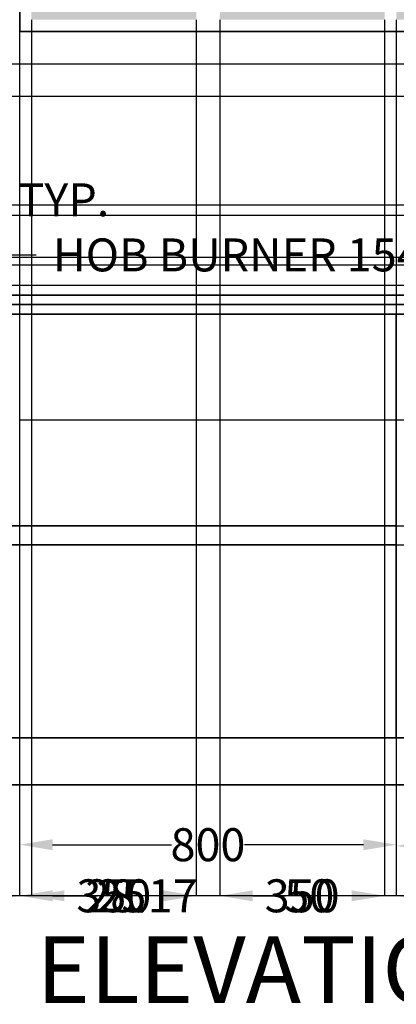
# Model space of a CAD drawing. Units: inches. Extents: x 600 to 5582, y -464 to 3142.
# Tile 7 of 9: x 3385 to 4185, y -464 to 1627. Entities that reach past the tile are written whole.
import ezdxf

# ---------------------------------------------------------------- set-up
doc = ezdxf.new("R2010")
doc.units = ezdxf.units.IN
doc.header["$MEASUREMENT"] = 0
for name, color, linetype, lineweight in [('A-ANNO-DIMS', 2, 'Continuous', 18), ('A-ANNO-TEXT', 7, 'Continuous', 25), ('A-ELEV', 7, 'Continuous', 35), ('A-ELEV-PATT', 252, 'Continuous', 13)]:
    doc.layers.add(name, color=color, linetype=linetype, lineweight=lineweight)
doc.styles.get("Standard").update_dxf_attribs({"font": 'arial.ttf'})
doc.dimstyles.get("Standard").update_dxf_attribs({"dimtxt": 70, "dimasz": 70, "dimexe": 0.18, "dimexo": 0.0625, "dimgap": 0.09, "dimtad": 0, "dimtih": 1, "dimtoh": 1, "dimdec": 0, "dimzin": 0, "dimdsep": 46, "dimtxsty": 'Standard', "dimcen": 0.09, "dimadec": 0, "dimazin": 0, "dimtfac": 1, "dimtdec": 0, "dimtofl": 0, "dimtmove": 0, "dimatfit": 3, "dimfxl": 1, "dimtolj": 1, "dimtzin": 0, "dimarcsym": 0})

# ---------------------------------------------------------------- blocks, each defined once
blk = doc.blocks.new('*D13')
at = {"layer": 'A-ANNO-DIMS', "color": 0, "lineweight": -2, "transparency": 16777216}
for p, q in [((3384.7, 2.4), (3384.7, -124.8)), ((4184.7, 2.4), (4184.7, -124.8)), ((3454.7, -124.6), (3707.4, -124.6)), ((4114.7, -124.6), (3862.1, -124.6))]:
    blk.add_line(p, q, dxfattribs=at)
at = {"layer": 'A-ANNO-DIMS', "color": 0, "transparency": 16777216}
for points in [[(3454.7, -113), (3454.7, -136.3), (3384.7, -124.6)], [(4114.7, -113), (4114.7, -136.3), (4184.7, -124.6)]]:
    blk.add_solid(points, dxfattribs=at)
at = {"layer": 'Defpoints', "color": 0, "transparency": 16777216}
for p in [(3384.7, 2.4), (4184.7, 2.4), (4184.7, -124.6)]:
    blk.add_point(p, dxfattribs=at)
at = {"layer": 'A-ANNO-DIMS', "color": 0, "transparency": 16777216, "insert": (3784.7, -124.6), "char_height": 70, "attachment_point": 5}
blk.add_mtext('\\A1;800', dxfattribs=at)
blk = doc.blocks.new('*D14')
at = {"layer": 'A-ANNO-DIMS', "color": 0, "lineweight": -2, "transparency": 16777216}
for p, q in [((4184.7, 2.4), (4184.7, -127.2)), ((4984.7, 2.4), (4984.7, -127.2)), ((4254.7, -127), (4507.4, -127)), ((4914.7, -127), (4662.1, -127))]:
    blk.add_line(p, q, dxfattribs=at)
at = {"layer": 'A-ANNO-DIMS', "color": 0, "transparency": 16777216}
for points in [[(4254.7, -115.3), (4254.7, -138.7), (4184.7, -127)], [(4914.7, -115.3), (4914.7, -138.7), (4984.7, -127)]]:
    blk.add_solid(points, dxfattribs=at)
at = {"layer": 'Defpoints', "color": 0, "transparency": 16777216}
for p in [(4184.7, 2.4), (4984.7, 2.4), (4984.7, -127)]:
    blk.add_point(p, dxfattribs=at)
at = {"layer": 'A-ANNO-DIMS', "color": 0, "transparency": 16777216, "insert": (4584.7, -127), "char_height": 70, "attachment_point": 5}
blk.add_mtext('\\A1;800', dxfattribs=at)
blk = doc.blocks.new('*D17')
at = {"layer": 'A-ANNO-DIMS', "color": 0, "lineweight": -2, "transparency": 16777216}
for p, q in [((3196.2, 1104.9), (3196.2, 1128.1)), ((3266.2, 1127.9), (3279.8, 1127.9)), ((3349.8, 1104.9), (3349.8, 1128.1)), ((3349.8, 1127.9), (3419.8, 1127.9))]:
    blk.add_line(p, q, dxfattribs=at)
at = {"layer": 'A-ANNO-DIMS', "color": 0, "transparency": 16777216}
for points in [[(3266.2, 1139.5), (3266.2, 1116.2), (3196.2, 1127.9)], [(3279.8, 1139.5), (3279.8, 1116.2), (3349.8, 1127.9)]]:
    blk.add_solid(points, dxfattribs=at)
at = {"layer": 'Defpoints', "color": 0, "transparency": 16777216}
for p in [(3349.8, 1127.9), (3196.2, 1104.9), (3349.8, 1104.9)]:
    blk.add_point(p, dxfattribs=at)
at = {"layer": 'A-ANNO-DIMS', "color": 0, "transparency": 16777216, "insert": (3955.1, 1127.9), "char_height": 70, "attachment_point": 5}
blk.add_mtext('\\A1;HOB BURNER 154 TYP.', dxfattribs=at)
blk = doc.blocks.new('*D18')
at = {"layer": 'A-ANNO-DIMS', "color": 0, "lineweight": -2, "transparency": 16777216}
for p, q in [((3173.2, 1174.9), (3173.2, 1244.9)), ((3173.2, 1244.9), (3243.2, 1244.9)), ((3196.2, 1104.9), (3173, 1104.9)), ((3196.2, 1042.4), (3173, 1042.4)), ((3173.2, 972.4), (3173.2, 902.4))]:
    blk.add_line(p, q, dxfattribs=at)
at = {"layer": 'A-ANNO-DIMS', "color": 0, "transparency": 16777216}
for points in [[(3161.5, 1174.9), (3184.9, 1174.9), (3173.2, 1104.9)], [(3161.5, 972.4), (3184.9, 972.4), (3173.2, 1042.4)]]:
    blk.add_solid(points, dxfattribs=at)
at = {"layer": 'Defpoints', "color": 0, "transparency": 16777216}
for p in [(3173.2, 1104.9), (3196.2, 1104.9), (3196.2, 1042.4)]:
    blk.add_point(p, dxfattribs=at)
at = {"layer": 'A-ANNO-DIMS', "color": 0, "transparency": 16777216, "insert": (3413.9, 1244.9), "char_height": 70, "attachment_point": 5}
blk.add_mtext('\\A1;62 TYP.', dxfattribs=at)
blk = doc.blocks.new('*D21')
at = {"layer": 'A-ANNO-DIMS', "color": 0, "lineweight": -2, "transparency": 16777216}
for p, q in [((1384.7, 2.4), (1384.7, -233.3)), ((4984.7, 2.4), (4984.7, -233.3)), ((1454.7, -233.1), (3080.3, -233.1)), ((4914.7, -233.1), (3289.2, -233.1))]:
    blk.add_line(p, q, dxfattribs=at)
at = {"layer": 'A-ANNO-DIMS', "color": 0, "transparency": 16777216}
for points in [[(1454.7, -221.4), (1454.7, -244.7), (1384.7, -233.1)], [(4914.7, -221.4), (4914.7, -244.7), (4984.7, -233.1)]]:
    blk.add_solid(points, dxfattribs=at)
at = {"layer": 'Defpoints', "color": 0, "transparency": 16777216}
for p in [(1384.7, 2.4), (4984.7, 2.4), (4984.7, -233.1)]:
    blk.add_point(p, dxfattribs=at)
at = {"layer": 'A-ANNO-DIMS', "color": 0, "transparency": 16777216, "insert": (3184.7, -233.1), "char_height": 70, "attachment_point": 5}
blk.add_mtext('\\A1;3600', dxfattribs=at)
blk = doc.blocks.new('*D26')
at = {"layer": 'A-ANNO-DIMS', "color": 0, "lineweight": -2, "transparency": 16777216}
for p, q in [((3409.7, 1627.4), (3409.7, -233.3)), ((3384.7, 1602.4), (3384.7, -233.3)), ((3314.7, -233.1), (3244.7, -233.1)), ((3479.7, -233.1), (3549.7, -233.1))]:
    blk.add_line(p, q, dxfattribs=at)
at = {"layer": 'A-ANNO-DIMS', "color": 0, "transparency": 16777216}
for points in [[(3314.7, -221.4), (3314.7, -244.7), (3384.7, -233.1)], [(3479.7, -221.4), (3479.7, -244.7), (3409.7, -233.1)]]:
    blk.add_solid(points, dxfattribs=at)
at = {"layer": 'Defpoints', "color": 0, "transparency": 16777216}
for p in [(3409.7, 1627.4), (3384.7, 1602.4), (3409.7, -233.1)]:
    blk.add_point(p, dxfattribs=at)
at = {"layer": 'A-ANNO-DIMS', "color": 0, "transparency": 16777216, "insert": (3600.8, -233.1), "char_height": 70, "attachment_point": 5}
blk.add_mtext('\\A1;25', dxfattribs=at)
blk = doc.blocks.new('*D27')
at = {"layer": 'A-ANNO-DIMS', "color": 0, "lineweight": -2, "transparency": 16777216}
for p, q in [((3409.7, 1627.4), (3409.7, -233.3)), ((3759.7, 1627.4), (3759.7, -233.3)), ((3479.7, -233.1), (3507.5, -233.1)), ((3689.7, -233.1), (3662, -233.1))]:
    blk.add_line(p, q, dxfattribs=at)
at = {"layer": 'A-ANNO-DIMS', "color": 0, "transparency": 16777216}
for points in [[(3479.7, -221.4), (3479.7, -244.7), (3409.7, -233.1)], [(3689.7, -221.4), (3689.7, -244.7), (3759.7, -233.1)]]:
    blk.add_solid(points, dxfattribs=at)
at = {"layer": 'Defpoints', "color": 0, "transparency": 16777216}
for p in [(3409.7, 1627.4), (3759.7, 1627.4), (3759.7, -233.1)]:
    blk.add_point(p, dxfattribs=at)
at = {"layer": 'A-ANNO-DIMS', "color": 0, "transparency": 16777216, "insert": (3584.7, -233.1), "char_height": 70, "attachment_point": 5}
blk.add_mtext('\\A1;350', dxfattribs=at)
blk = doc.blocks.new('*D28')
at = {"layer": 'A-ANNO-DIMS', "color": 0, "lineweight": -2, "transparency": 16777216}
for p, q in [((3759.7, 1627.4), (3759.7, -233.3)), ((3809.7, 1627.4), (3809.7, -233.3)), ((3689.7, -233.1), (3619.7, -233.1)), ((3879.7, -233.1), (3949.7, -233.1))]:
    blk.add_line(p, q, dxfattribs=at)
at = {"layer": 'A-ANNO-DIMS', "color": 0, "transparency": 16777216}
for points in [[(3689.7, -221.4), (3689.7, -244.7), (3759.7, -233.1)], [(3879.7, -221.4), (3879.7, -244.7), (3809.7, -233.1)]]:
    blk.add_solid(points, dxfattribs=at)
at = {"layer": 'Defpoints', "color": 0, "transparency": 16777216}
for p in [(3759.7, 1627.4), (3809.7, 1627.4), (3809.7, -233.1)]:
    blk.add_point(p, dxfattribs=at)
at = {"layer": 'A-ANNO-DIMS', "color": 0, "transparency": 16777216, "insert": (3999.9, -233.1), "char_height": 70, "attachment_point": 5}
blk.add_mtext('\\A1;50', dxfattribs=at)
blk = doc.blocks.new('*D29')
at = {"layer": 'A-ANNO-DIMS', "color": 0, "lineweight": -2, "transparency": 16777216}
for p, q in [((3809.7, 1627.4), (3809.7, -233.3)), ((4159.7, 1627.4), (4159.7, -233.3)), ((3879.7, -233.1), (3907.5, -233.1)), ((4089.7, -233.1), (4062, -233.1))]:
    blk.add_line(p, q, dxfattribs=at)
at = {"layer": 'A-ANNO-DIMS', "color": 0, "transparency": 16777216}
for points in [[(3879.7, -221.4), (3879.7, -244.7), (3809.7, -233.1)], [(4089.7, -221.4), (4089.7, -244.7), (4159.7, -233.1)]]:
    blk.add_solid(points, dxfattribs=at)
at = {"layer": 'Defpoints', "color": 0, "transparency": 16777216}
for p in [(3809.7, 1627.4), (4159.7, 1627.4), (4159.7, -233.1)]:
    blk.add_point(p, dxfattribs=at)
at = {"layer": 'A-ANNO-DIMS', "color": 0, "transparency": 16777216, "insert": (3984.7, -233.1), "char_height": 70, "attachment_point": 5}
blk.add_mtext('\\A1;350', dxfattribs=at)
blk = doc.blocks.new('*D30')
at = {"layer": 'A-ANNO-DIMS', "color": 0, "lineweight": -2, "transparency": 16777216}
for p, q in [((4159.7, 1627.4), (4159.7, -233.3)), ((4184.7, 1627.4), (4184.7, -233.3)), ((4089.7, -233.1), (4019.7, -233.1)), ((4254.7, -233.1), (4324.7, -233.1))]:
    blk.add_line(p, q, dxfattribs=at)
at = {"layer": 'A-ANNO-DIMS', "color": 0, "transparency": 16777216}
for points in [[(4089.7, -221.4), (4089.7, -244.7), (4159.7, -233.1)], [(4254.7, -221.4), (4254.7, -244.7), (4184.7, -233.1)]]:
    blk.add_solid(points, dxfattribs=at)
at = {"layer": 'Defpoints', "color": 0, "transparency": 16777216}
for p in [(4159.7, 1627.4), (4184.7, 1627.4), (4184.7, -233.1)]:
    blk.add_point(p, dxfattribs=at)
at = {"layer": 'A-ANNO-DIMS', "color": 0, "transparency": 16777216, "insert": (4375.8, -233.1), "char_height": 70, "attachment_point": 5}
blk.add_mtext('\\A1;25', dxfattribs=at)
blk = doc.blocks.new('*D47')
at = {"layer": 'A-ANNO-DIMS', "color": 0, "lineweight": -2, "transparency": 16777216}
for p, q in [((3384.8, 1002.4), (5220.4, 1002.4)), ((5220.2, 932.4), (5220.2, 925.8)), ((5220.2, 847.4), (5220.2, 854.1)), ((3384.8, 777.4), (5220.4, 777.4))]:
    blk.add_line(p, q, dxfattribs=at)
at = {"layer": 'A-ANNO-DIMS', "color": 0, "transparency": 16777216}
for points in [[(5208.6, 932.4), (5231.9, 932.4), (5220.2, 1002.4)], [(5208.6, 847.4), (5231.9, 847.4), (5220.2, 777.4)]]:
    blk.add_solid(points, dxfattribs=at)
at = {"layer": 'Defpoints', "color": 0, "transparency": 16777216}
for p in [(3384.7, 1002.4), (5220.2, 1002.4), (3384.7, 777.4)]:
    blk.add_point(p, dxfattribs=at)
at = {"layer": 'A-ANNO-DIMS', "color": 0, "transparency": 16777216, "insert": (5220.2, 889.9), "char_height": 70, "attachment_point": 5}
blk.add_mtext('\\A1;225', dxfattribs=at)
blk = doc.blocks.new('*D56')
at = {"layer": 'A-ANNO-DIMS', "color": 0, "lineweight": -2, "transparency": 16777216}
for p, q in [((1884.8, 512.4), (5220.4, 512.4)), ((5220.2, 442.4), (5220.2, 343.3)), ((5220.2, 172.4), (5220.2, 271.6)), ((1884.8, 102.4), (5220.4, 102.4))]:
    blk.add_line(p, q, dxfattribs=at)
at = {"layer": 'A-ANNO-DIMS', "color": 0, "transparency": 16777216}
for points in [[(5208.6, 442.4), (5231.9, 442.4), (5220.2, 512.4)], [(5208.6, 172.4), (5231.9, 172.4), (5220.2, 102.4)]]:
    blk.add_solid(points, dxfattribs=at)
at = {"layer": 'Defpoints', "color": 0, "transparency": 16777216}
for p in [(1884.7, 512.4), (5220.2, 512.4), (1884.7, 102.4)]:
    blk.add_point(p, dxfattribs=at)
at = {"layer": 'A-ANNO-DIMS', "color": 0, "transparency": 16777216, "insert": (5220.2, 307.4), "char_height": 70, "attachment_point": 5}
blk.add_mtext('\\A1;410', dxfattribs=at)
blk = doc.blocks.new('*D57')
at = {"layer": 'A-ANNO-DIMS', "color": 0, "lineweight": -2, "transparency": 16777216}
for p, q in [((5220.2, 622.4), (5220.2, 692.4)), ((5220.2, 692.4), (5290.2, 692.4)), ((1884.8, 552.4), (5220.4, 552.4)), ((1884.8, 512.4), (5220.4, 512.4)), ((5220.2, 442.4), (5220.2, 372.4))]:
    blk.add_line(p, q, dxfattribs=at)
at = {"layer": 'A-ANNO-DIMS', "color": 0, "transparency": 16777216}
for points in [[(5208.6, 622.4), (5231.9, 622.4), (5220.2, 552.4)], [(5208.6, 442.4), (5231.9, 442.4), (5220.2, 512.4)]]:
    blk.add_solid(points, dxfattribs=at)
at = {"layer": 'Defpoints', "color": 0, "transparency": 16777216}
for p in [(1884.7, 552.4), (5220.2, 552.4), (1884.7, 512.4)]:
    blk.add_point(p, dxfattribs=at)
at = {"layer": 'A-ANNO-DIMS', "color": 0, "transparency": 16777216, "insert": (5341.8, 692.4), "char_height": 70, "attachment_point": 5}
blk.add_mtext('\\A1;40', dxfattribs=at)
blk = doc.blocks.new('*D64')
at = {"layer": 'A-ANNO-DIMS', "color": 0, "lineweight": -2, "transparency": 16777216}
for p, q in [((3384.7, 1680.8), (3384.7, -233.3)), ((3356.6, 1655.8), (3356.6, -233.3)), ((3286.6, -233.1), (3216.6, -233.1)), ((3454.7, -233.1), (3524.7, -233.1))]:
    blk.add_line(p, q, dxfattribs=at)
at = {"layer": 'A-ANNO-DIMS', "color": 0, "transparency": 16777216}
for points in [[(3286.6, -221.4), (3286.6, -244.7), (3356.6, -233.1)], [(3454.7, -221.4), (3454.7, -244.7), (3384.7, -233.1)]]:
    blk.add_solid(points, dxfattribs=at)
at = {"layer": 'Defpoints', "color": 0, "transparency": 16777216}
for p in [(3384.7, 1680.8), (3356.6, 1655.8), (3384.7, -233.1)]:
    blk.add_point(p, dxfattribs=at)
at = {"layer": 'A-ANNO-DIMS', "color": 0, "transparency": 16777216, "insert": (3643.5, -233.1), "char_height": 70, "attachment_point": 5}
blk.add_mtext('\\A1;28.17', dxfattribs=at)
blk = doc.blocks.new('*D69')
at = {"layer": 'A-ANNO-DIMS', "color": 0, "lineweight": -2, "transparency": 16777216}
for p, q in [((5220.2, 1304), (5220.2, 1374)), ((2777.3, 1234), (5220.4, 1234)), ((2777.3, 1106.8), (5220.4, 1106.8)), ((5220.2, 1036.8), (5220.2, 966.8))]:
    blk.add_line(p, q, dxfattribs=at)
at = {"layer": 'A-ANNO-DIMS', "color": 0, "transparency": 16777216}
for points in [[(5208.6, 1304), (5231.9, 1304), (5220.2, 1234)], [(5208.6, 1036.8), (5231.9, 1036.8), (5220.2, 1106.8)]]:
    blk.add_solid(points, dxfattribs=at)
at = {"layer": 'Defpoints', "color": 0, "transparency": 16777216}
for p in [(2777.3, 1234), (5220.2, 1234), (2777.3, 1106.8)]:
    blk.add_point(p, dxfattribs=at)
at = {"layer": 'A-ANNO-DIMS', "color": 0, "transparency": 16777216, "insert": (5220.2, 1170.4), "char_height": 70, "attachment_point": 5}
blk.add_mtext('\\A1;127.21', dxfattribs=at)
blk = doc.blocks.new('*D72')
at = {"layer": 'A-ANNO-DIMS', "color": 0, "lineweight": -2, "transparency": 16777216}
for p, q in [((5220.2, 1304), (5220.2, 1374)), ((5220.2, 1374), (5290.2, 1374)), ((2947.9, 1234), (5220.4, 1234)), ((2947.9, 1212), (5220.4, 1212)), ((5220.2, 1142), (5220.2, 1072))]:
    blk.add_line(p, q, dxfattribs=at)
at = {"layer": 'A-ANNO-DIMS', "color": 0, "transparency": 16777216}
for points in [[(5208.6, 1304), (5231.9, 1304), (5220.2, 1234)], [(5208.6, 1142), (5231.9, 1142), (5220.2, 1212)]]:
    blk.add_solid(points, dxfattribs=at)
at = {"layer": 'Defpoints', "color": 0, "transparency": 16777216}
for p in [(2947.8, 1234), (5220.2, 1234), (2947.8, 1212)]:
    blk.add_point(p, dxfattribs=at)
at = {"layer": 'A-ANNO-DIMS', "color": 0, "transparency": 16777216, "insert": (5436.2, 1374), "char_height": 70, "attachment_point": 5}
blk.add_mtext('\\A1;22.087', dxfattribs=at)
blk = doc.blocks.new('*D81')
at = {"layer": 'A-ANNO-DIMS', "color": 0, "lineweight": -2, "transparency": 16777216}
for p, q in [((5220.2, 1133.7), (5220.2, 1203.7)), ((5220.2, 1203.7), (5290.2, 1203.7)), ((2292.1, 1063.7), (5220.4, 1063.7)), ((2310.1, 1042.4), (5220.4, 1042.4)), ((5220.2, 972.4), (5220.2, 902.4))]:
    blk.add_line(p, q, dxfattribs=at)
at = {"layer": 'A-ANNO-DIMS', "color": 0, "transparency": 16777216}
for points in [[(5208.6, 1133.7), (5231.9, 1133.7), (5220.2, 1063.7)], [(5208.6, 972.4), (5231.9, 972.4), (5220.2, 1042.4)]]:
    blk.add_solid(points, dxfattribs=at)
at = {"layer": 'Defpoints', "color": 0, "transparency": 16777216}
for p in [(2292, 1063.7), (5220.2, 1063.7), (2310, 1042.4)]:
    blk.add_point(p, dxfattribs=at)
at = {"layer": 'A-ANNO-DIMS', "color": 0, "transparency": 16777216, "insert": (5409, 1203.7), "char_height": 70, "attachment_point": 5}
blk.add_mtext('\\A1;21.26', dxfattribs=at)
blk = doc.blocks.new('*D85')
at = {"layer": 'A-ANNO-DIMS', "color": 0, "lineweight": -2, "transparency": 16777216}
for p, q in [((5220.2, 1193.3), (5220.2, 1263.3)), ((5220.2, 1263.3), (5290.2, 1263.3)), ((2231.9, 1123.3), (5220.4, 1123.3)), ((2232.3, 1063.4), (5220.4, 1063.4)), ((5220.2, 993.4), (5220.2, 923.4))]:
    blk.add_line(p, q, dxfattribs=at)
at = {"layer": 'A-ANNO-DIMS', "color": 0, "transparency": 16777216}
for points in [[(5208.6, 1193.3), (5231.9, 1193.3), (5220.2, 1123.3)], [(5208.6, 993.4), (5231.9, 993.4), (5220.2, 1063.4)]]:
    blk.add_solid(points, dxfattribs=at)
at = {"layer": 'Defpoints', "color": 0, "transparency": 16777216}
for p in [(2231.8, 1123.3), (5220.2, 1123.3), (2232.2, 1063.4)]:
    blk.add_point(p, dxfattribs=at)
at = {"layer": 'A-ANNO-DIMS', "color": 0, "transparency": 16777216, "insert": (5408.5, 1263.3), "char_height": 70, "attachment_point": 5}
blk.add_mtext('\\A1;59.99', dxfattribs=at)
blk = doc.blocks.new('*D99')
at = {"layer": 'A-ANNO-DIMS', "color": 0, "lineweight": -2, "transparency": 16777216}
for p, q in [((5220.2, 1603.5), (5220.2, 1673.5)), ((2271, 1533.5), (5220.4, 1533.5)), ((2273, 1464.8), (5220.4, 1464.8)), ((5220.2, 1394.8), (5220.2, 1324.8)), ((5220.2, 1324.8), (5150.2, 1324.8))]:
    blk.add_line(p, q, dxfattribs=at)
at = {"layer": 'A-ANNO-DIMS', "color": 0, "transparency": 16777216}
for points in [[(5208.6, 1603.5), (5231.9, 1603.5), (5220.2, 1533.5)], [(5208.6, 1394.8), (5231.9, 1394.8), (5220.2, 1464.8)]]:
    blk.add_solid(points, dxfattribs=at)
at = {"layer": 'Defpoints', "color": 0, "transparency": 16777216}
for p in [(2271, 1533.5), (2272.9, 1464.8), (5220.2, 1464.8)]:
    blk.add_point(p, dxfattribs=at)
at = {"layer": 'A-ANNO-DIMS', "color": 0, "transparency": 16777216, "insert": (5038.6, 1324.8), "char_height": 70, "attachment_point": 5}
blk.add_mtext('\\A1;68.71', dxfattribs=at)

msp = doc.modelspace()

# ---------------------------------------------------------------- hatches: boundary and pattern name
at = {"layer": 'A-ELEV-PATT'}
h = msp.add_hatch(dxfattribs=at)
h.set_pattern_fill('GOST_WOOD', color=256, scale=15)
h.set_pattern_definition([(90, (0, 0), (90, -6e-15), [150, -30]), (90, (30, -30), (90, -6e-15), [90, -22.5, 45, -22.5]), (90, (60, -75), (90, -6e-15), [150, -30])])
h.paths.add_polyline_path([(4959.7485, 2752.4212), (1409.7485, 2752.4212), (1409.7485, 2352.4212), (1784.7485, 2352.4212), (4959.7485, 2352.4212)])
h.paths.add_polyline_path([(3384.7485, 1002.4212), (2584.7485, 1002.4212), (2584.7485, 777.4212), (3384.7485, 777.4212)])
h.paths.add_polyline_path([(3384.7485, 777.4212), (2584.7485, 777.4212), (2584.7485, 552.4212), (3384.7485, 552.4212)])
h.paths.add_polyline_path([(3384.7485, 512.4212), (2584.7485, 512.4212), (2584.7485, 102.4212), (3384.7485, 102.4212)])
h = msp.add_hatch(dxfattribs=at)
h.set_pattern_fill('CROSS', color=256, scale=100)
h.paths.add_polyline_path([(1759.7485, 2327.4212), (1409.7485, 2327.4212), (1409.7485, 1967.4212), (1759.7485, 1967.4212)])
h.paths.add_polyline_path([(1759.7485, 1952.4212), (1409.7485, 1952.4212), (1409.7485, 1567.4212), (1759.7485, 1567.4212)])
h.paths.add_polyline_path([(1759.7485, 1552.4212), (1409.7485, 1552.4212), (1409.7485, 1167.4212), (1759.7485, 1167.4212)])
h.paths.add_polyline_path([(1759.7485, 1152.4212), (1409.7485, 1152.4212), (1409.7485, 767.4212), (1759.7485, 767.4212)])
h.paths.add_polyline_path([(1759.7485, 752.4212), (1409.7485, 752.4212), (1409.7485, 367.4212), (1759.7485, 367.4212)])
h.paths.add_polyline_path([(1759.7485, 352.4212), (1409.7485, 352.4212), (1409.7485, 142.4212), (1759.7485, 142.4212)])
h.paths.add_polyline_path([(3759.7485, 1977.4212), (3409.7485, 1977.4212), (3409.7485, 1627.4212), (3759.7485, 1627.4212)])
h.paths.add_polyline_path([(3714.7508, 1954.858, -1), (3750.8891, 1954.858, -1)], flags=16)
h.paths.add_polyline_path([(3759.7485, 2327.4212), (3409.7485, 2327.4212), (3409.7485, 2002.4212), (3759.7485, 2002.4212)])
h.paths.add_polyline_path([(4159.7485, 2327.4212), (3809.7485, 2327.4212), (3809.7485, 2002.4212), (4159.7485, 2002.4212)])
h.paths.add_polyline_path([(4159.7485, 1977.4212), (3809.7485, 1977.4212), (3813.5467, 1954.858, -1), (3849.685, 1954.858, -1), (3813.5467, 1954.858), (3809.7485, 1627.4212), (4159.7485, 1627.4212)])
h.paths.add_polyline_path([(4559.7485, 2327.4212), (4184.7485, 2327.4212), (4184.7485, 2002.4212), (4559.7485, 2002.4212)])
h.paths.add_polyline_path([(4559.7485, 1977.4212), (4184.7485, 1977.4212), (4184.7485, 1627.4212), (4559.7485, 1627.4212)])
h.paths.add_polyline_path([(4517.0704, 1954.858, -1), (4553.2087, 1954.858, -1)], flags=16)
h.paths.add_polyline_path([(4959.7485, 2327.4212), (4609.7485, 2327.4212), (4609.7485, 2002.4212), (4959.7485, 2002.4212)])
h.paths.add_polyline_path([(4959.7485, 1977.4212), (4609.7485, 1977.4212), (4609.7485, 1627.4212), (4959.7485, 1627.4212)])
h.paths.add_polyline_path([(4619.5464, 1954.858, -1), (4655.6847, 1954.858, -1)], flags=16)

# ---------------------------------------------------------------- linework, layer by layer
at = {"layer": 'A-ELEV'}
for p, q in [((4984.7485, 1042.4212), (1784.7485, 1042.4212)), ((4984.7485, 1022.4212), (1784.7485, 1022.4212)), ((4984.7485, 1002.4212), (1784.7485, 1002.4212)), ((4184.7485, 102.4212), (4184.7485, 1002.4212)), ((4184.7485, 552.4212), (1884.7485, 552.4212)), ((4184.7485, 512.4212), (1884.7485, 512.4212)), ((4984.7485, 102.4212), (1384.7485, 102.4212))]:
    msp.add_line(p, q, dxfattribs=at)
msp.add_lwpolyline([(4984.7485, 2.4212), (4984.7485, 2752.4212), (1384.7485, 2752.4212), (1384.7485, 2.4212)], close=True, dxfattribs=at)
msp.add_lwpolyline([(4984.7485, 1602.4212), (3384.7485, 1602.4212), (3384.7485, 2352.4212), (3784.7485, 2352.4212)], dxfattribs=at)

# ---------------------------------------------------------------- texts
at = {"layer": 'A-ANNO-TEXT'}
msp.add_text('MODULAR KITCHEN ELEVATION', height=141.903549, dxfattribs=at).set_placement((1598.0156, -460.987))

# ---------------------------------------------------------------- dimensions: what is measured, and where the dimension line sits
at = {"layer": 'A-ANNO-DIMS'}
for base, p1, p2, override, picture, middle in [((5220.2485, 1464.7817), (2270.9593, 1533.4874), (2272.9025, 1464.7817), {"dimdec": 2, "dimlfac": 1, "dimrnd": 0, "dimzin": 0, "dimdsep": 46, "dimlunit": 2}, '*D99', (5038.6169, 1324.7817)), ((5220.2485, 1234.0488), (2947.8448, 1211.9616), (2947.8448, 1234.0488), {"dimdec": 3, "dimlfac": 1, "dimrnd": 0, "dimzin": 0, "dimdsep": 46, "dimlunit": 2}, '*D72', (5436.2355, 1374.0488)), ((5220.2485, 1234.0488), (2777.2556, 1106.8415), (2777.2556, 1234.0488), {"dimdec": 2, "dimlfac": 1, "dimrnd": 0, "dimzin": 0, "dimdsep": 46, "dimlunit": 2}, '*D69', (5220.2485, 1170.4451)), ((5220.2485, 1123.3472), (2232.228, 1063.362), (2231.8275, 1123.3472), {"dimdec": 2, "dimlfac": 1, "dimrnd": 0, "dimzin": 0, "dimdsep": 46, "dimlunit": 2}, '*D85', (5408.5172, 1263.3472)), ((5220.2485, 1063.682), (2310.0444, 1042.4212), (2292.0448, 1063.682), {"dimdec": 2, "dimlfac": 1, "dimrnd": 0, "dimzin": 0, "dimdsep": 46, "dimlunit": 2}, '*D81', (5409.0186, 1203.682)), ((5220.2485, 1002.4212), (3384.7485, 777.4212), (3384.7485, 1002.4212), {"dimdec": 0, "dimlfac": 1, "dimrnd": 0, "dimzin": 0, "dimdsep": 46, "dimlunit": 2}, '*D47', (5220.2485, 889.9212)), ((5220.2485, 552.4212), (1884.7485, 512.4212), (1884.7485, 552.4212), {"dimdec": 0, "dimlfac": 1, "dimrnd": 0, "dimzin": 0, "dimdsep": 46, "dimlunit": 2}, '*D57', (5341.7641, 692.4212)), ((5220.2485, 512.4212), (1884.7485, 102.4212), (1884.7485, 512.4212), {"dimdec": 0, "dimlfac": 1, "dimrnd": 0, "dimzin": 0, "dimdsep": 46, "dimlunit": 2}, '*D56', (5220.2485, 307.4212))]:
    dim = msp.add_linear_dim(base=base, p1=p1, p2=p2, angle=90, dimstyle='Standard', override=override, dxfattribs=at)
    dim.commit()
    dim.dimension.update_dxf_attribs({"geometry": picture, "text_midpoint": middle})
for base, p1, p2, override, picture, middle in [((3384.7485, -233.0788), (3356.5781, 1655.8271), (3384.7485, 1680.8271), {"dimdec": 2, "dimlfac": 1, "dimrnd": 0, "dimzin": 0, "dimdsep": 46, "dimlunit": 2}, '*D64', (3643.5424, -233.0788)), ((3409.7485, -233.0788), (3384.7485, 1602.4212), (3409.7485, 1627.4212), {"dimdec": 0, "dimlfac": 1, "dimrnd": 0, "dimzin": 0, "dimdsep": 46, "dimlunit": 2}, '*D26', (3600.8344, -233.0788)), ((3759.7485, -233.0788), (3409.7485, 1627.4212), (3759.7485, 1627.4212), {"dimdec": 0, "dimlfac": 1, "dimrnd": 0, "dimzin": 0, "dimdsep": 46, "dimlunit": 2}, '*D27', (3584.7485, -233.0788)), ((3809.7485, -233.0788), (3759.7485, 1627.4212), (3809.7485, 1627.4212), {"dimdec": 0, "dimlfac": 1, "dimrnd": 0, "dimzin": 0, "dimdsep": 46, "dimlunit": 2}, '*D28', (3999.8555, -233.0788)), ((4159.7485, -233.0788), (3809.7485, 1627.4212), (4159.7485, 1627.4212), {"dimdec": 0, "dimlfac": 1, "dimrnd": 0, "dimzin": 0, "dimdsep": 46, "dimlunit": 2}, '*D29', (3984.7485, -233.0788)), ((4184.7485, -233.0788), (4159.7485, 1627.4212), (4184.7485, 1627.4212), {"dimdec": 0, "dimlfac": 1, "dimrnd": 0, "dimzin": 0, "dimdsep": 46, "dimlunit": 2}, '*D30', (4375.8344, -233.0788)), ((4984.7485, -233.0788), (1384.7485, 2.4212), (4984.7485, 2.4212), {"dimdec": 0, "dimlfac": 1, "dimrnd": 0, "dimzin": 0, "dimdsep": 46, "dimlunit": 2}, '*D21', (3184.7485, -233.0788)), ((4184.7485, -124.6307), (3384.7485, 2.4212), (4184.7485, 2.4212), {"dimclrd": 0, "dimclre": 0, "dimclrt": 0}, '*D13', (3784.7485, -124.6307)), ((4984.7485, -126.996), (4184.7485, 2.4212), (4984.7485, 2.4212), {"dimclrd": 0, "dimclre": 0, "dimclrt": 0}, '*D14', (4584.7485, -126.996))]:
    dim = msp.add_linear_dim(base=base, p1=p1, p2=p2, dimstyle='Standard', override=override, dxfattribs=at)
    dim.commit()
    dim.dimension.update_dxf_attribs({"geometry": picture, "text_midpoint": middle})
dim = msp.add_linear_dim(base=(3173.2092, 1104.8519), p1=(3196.2381, 1042.4212), p2=(3196.2381, 1104.8519), angle=90, text='<> TYP.', dimstyle='Standard', override={"dimdec": 0, "dimrnd": 0, "dimzin": 0, "dimlunit": 2}, dxfattribs=at)
dim.commit()
dim.dimension.update_dxf_attribs({"geometry": '*D18', "text_midpoint": (3413.8585, 1244.8519)})
dim = msp.add_linear_dim(base=(3349.7642, 1127.8808), p1=(3196.2381, 1104.8519), p2=(3349.7642, 1104.8519), text='HOB BURNER <> TYP.', dimstyle='Standard', override={"dimdec": 0, "dimrnd": 0, "dimzin": 0, "dimlunit": 2}, dxfattribs=at)
dim.commit()
dim.dimension.update_dxf_attribs({"geometry": '*D17', "text_midpoint": (3955.1203, 1127.8808)})

doc.saveas('drawing.dxf')
